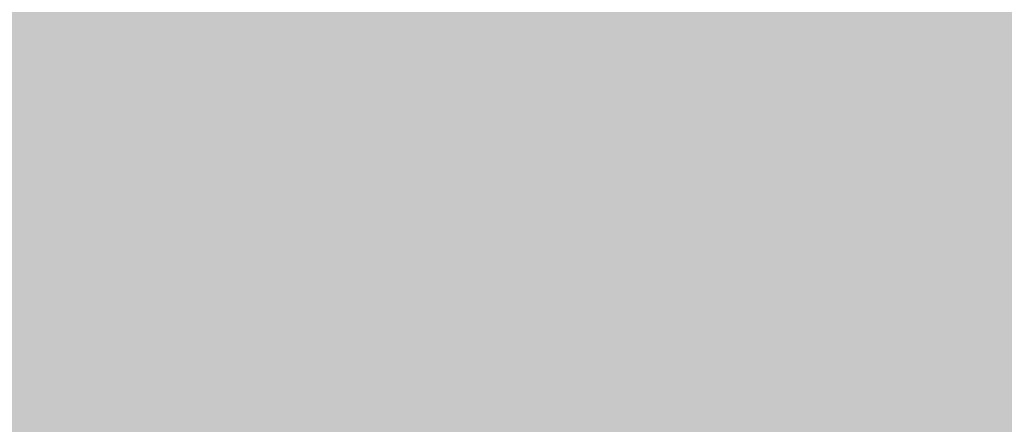
# Model space of a CAD drawing. Units: feet. Extents: x 3168 to 4724, y 827 to 1477.
# Tile 203 of 256: x 3333 to 3364, y 1075 to 1087. Entities that reach past the tile are written whole.
import ezdxf

# ---------------------------------------------------------------- set-up
doc = ezdxf.new("R2010")
doc.units = ezdxf.units.FT
doc.layers.add('A-ELEV-PATT', color=8, linetype='Continuous', lineweight=13)

msp = doc.modelspace()

# ---------------------------------------------------------------- hatches: boundary and pattern name
at = {"layer": 'A-ELEV-PATT'}
h = msp.add_hatch(color=256, dxfattribs=at)
h.dxf.hatch_style = 1
edge = h.paths.add_edge_path()
edge.add_ellipse((3552.906, 979.22), major_axis=(36.745, 0), ratio=0.484848, start_angle=0, end_angle=360)
edge = h.paths.add_edge_path()
edge.add_ellipse((3559.892, 929.252), major_axis=(36.745, 0), ratio=0.484848, start_angle=0, end_angle=360)
edge = h.paths.add_edge_path()
edge.add_line((3299.317, 1198.606), (3479.917, 1198.606))
edge.add_line((3479.917, 1198.606), (3479.917, 1209.869))
edge.add_spline(control_points=[(3479.917, 1209.869), (3464.301, 1209.869), (3448.686, 1209.869), (3410.949, 1209.869), (3388.828, 1209.869), (3355.647, 1209.869), (3344.586, 1209.869), (3327.996, 1209.869), (3322.466, 1209.869), (3314.17, 1209.869), (3311.405, 1209.869), (3307.257, 1209.869), (3305.875, 1209.869), (3303.801, 1209.869), (3303.11, 1209.869), (3302.073, 1209.869), (3301.727, 1209.869), (3301.209, 1209.869), (3301.036, 1209.869), (3300.777, 1209.869), (3300.69, 1209.869), (3300.561, 1209.869), (3300.517, 1209.869), (3300.453, 1209.869), (3300.431, 1209.869), (3300.399, 1209.869), (3300.388, 1209.869), (3300.366, 1209.869), (3300.346, 1209.869), (3300.346, 1209.869), (3300.346, 1209.869), (3300.343, 1209.869), (3300.341, 1209.869), (3300.338, 1209.869), (3300.337, 1209.869), (3300.334, 1209.869), (3300.332, 1209.869), (3300.326, 1209.869), (3300.321, 1209.869), (3300.311, 1209.869), (3300.306, 1209.869), (3300.291, 1209.869), (3300.28, 1209.869), (3300.232, 1209.869), (3300.195, 1209.869), (3299.951, 1209.871), (3299.745, 1209.874), (3299.437, 1209.883), (3299.334, 1209.887), (3299.181, 1209.893), (3299.13, 1209.895), (3298.652, 1209.917), (3298.229, 1209.946), (3297.602, 1210.002), (3297.393, 1210.023), (3297.083, 1210.058), (3296.979, 1210.07), (3296.293, 1210.155), (3295.718, 1210.243), (3294.869, 1210.399), (3294.588, 1210.454), (3294.169, 1210.543), (3294.03, 1210.574), (3291.707, 1211.101), (3289.654, 1211.813), (3285.776, 1213.564), (3283.951, 1214.603), (3280.512, 1216.98), (3278.897, 1218.318), (3276.38, 1220.829), (3275.416, 1221.918), (3274.039, 1223.708), (3273.581, 1224.35), (3273.143, 1225.016)], knot_values=[39.119033, 39.119033, 39.119033, 39.119033, 39.286353, 39.286353, 39.523379, 39.523379, 39.641892, 39.641892, 39.701148, 39.701148, 39.730777, 39.730777, 39.745591, 39.745591, 39.752998, 39.752998, 39.756701, 39.756701, 39.758553, 39.758553, 39.759479, 39.759479, 39.759942, 39.759942, 39.760173, 39.760173, 39.760289, 39.760289, 39.760405, 39.760405, 39.760463, 39.760463, 39.763389, 39.763389, 39.764851, 39.764851, 39.767304, 39.767304, 39.773825, 39.773825, 39.78057, 39.78057, 39.79477, 39.79477, 39.845194, 39.845194, 40.126715, 40.126715, 40.267476, 40.267476, 40.337856, 40.337856, 40.927023, 40.927023, 41.221606, 41.221606, 41.368898, 41.368898, 42.202622, 42.202622, 42.619485, 42.619485, 42.827916, 42.827916, 46.118323, 46.118323, 49.408731, 49.408731, 52.699139, 52.699139, 54.927489, 54.927489, 56.104228, 56.104228, 56.104228, 56.104228], weights=[1, 1, 1, 1, 1, 1, 1, 1, 1, 1, 1, 1, 1, 1, 1, 1, 1, 1, 1, 1, 1, 1, 1, 1, 1, 1, 1, 1, 1, 1, 1, 1, 1, 1, 1, 1, 1, 1, 1, 1, 1, 1, 1, 1, 1, 1, 1, 1, 1, 1, 1, 1, 1, 1, 1, 1, 1, 1, 1, 1, 1, 1, 1, 1, 1, 1, 1, 1, 1, 1, 1, 1, 1, 1], degree=3, periodic=0)
edge.add_line((3273.143, 1225.016), (3273.143, 1099.016))
edge.add_line((3273.143, 1099.016), (3299.317, 1099.016))
edge.add_line((3299.317, 1099.016), (3299.317, 1198.606))
edge = h.paths.add_edge_path()
edge.add_line((3304.758, 1324.158), (3479.917, 1324.158))
edge.add_line((3479.917, 1324.158), (3479.917, 1335.715))
edge.add_line((3479.917, 1335.715), (3269.162, 1335.715))
edge.add_spline(control_points=[(3269.162, 1335.715), (3264.024, 1335.715), (3258.364, 1328.958), (3259.264, 1323.9)], knot_values=[0, 0, 0, 0, 15.412191, 15.412191, 15.412191, 15.412191], degree=3, periodic=0)
edge.add_line((3259.264, 1323.9), (3265.517, 1288.769))
edge.add_line((3265.517, 1288.769), (3275.265, 1261.546))
edge.add_line((3275.265, 1261.546), (3304.758, 1261.546))
edge.add_line((3304.758, 1261.546), (3304.758, 1324.158))
h = msp.add_hatch(color=256, dxfattribs=at)
h.dxf.hatch_style = 1
h.paths.add_polyline_path([(3384.525, 1099.016), (3335.029, 1099.016), (3299.317, 1099.016), (3273.143, 1099.016), (3217.565, 1099.016), (3168.069, 827.116), (3335.029, 827.116)])

doc.saveas('drawing.dxf')
